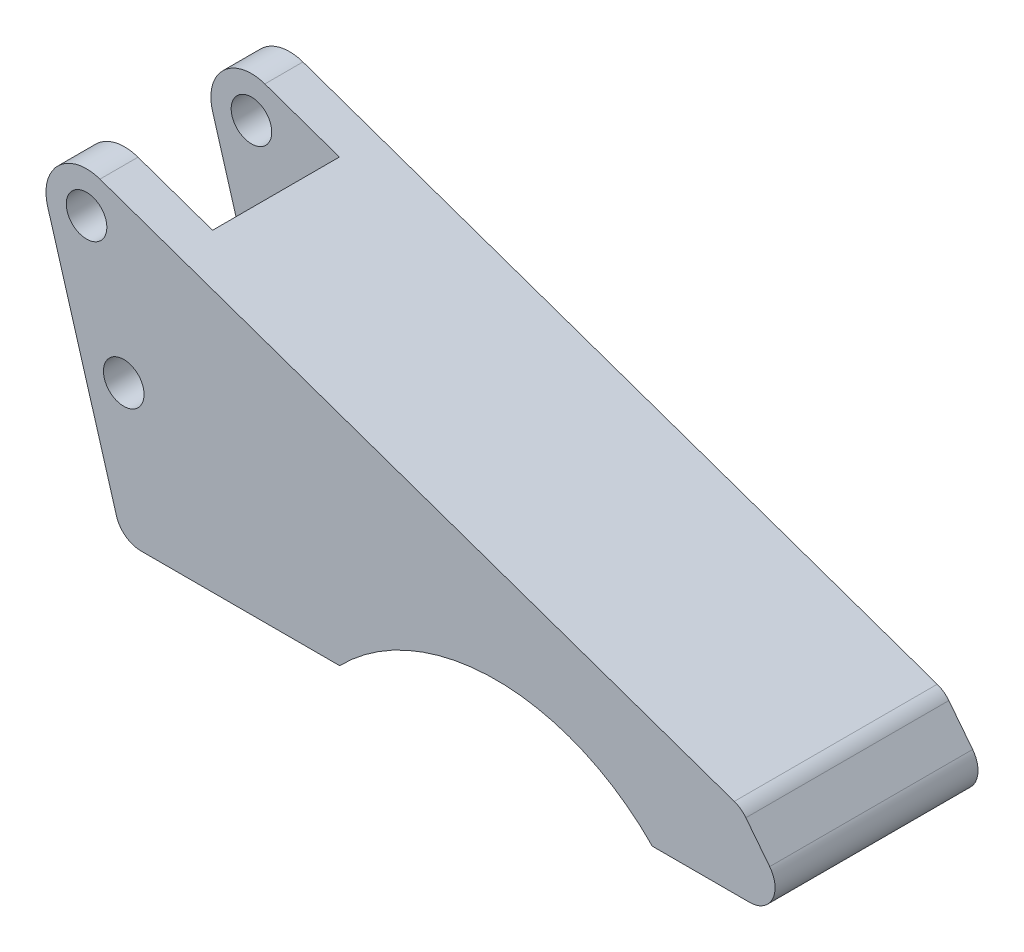
SolidWorks part; units mm, degrees
material "Plain Carbon Steel"
ref_plane "Front Plane" through (0, 0, 0) normal (0, 0, 1) x (1, 0, 0)
ref_plane "Top Plane" through (0, 0, 0) normal (0, 1, 0) x (1, 0, 0)
ref_plane "Right Plane" through (0, 0, 0) normal (1, 0, 0) x (0, 0, -1)
sketch "Jaw Profile Sketch" plane through (0, 0, 0) normal (0, 0, 1) x (1, 0, 0)
  line L0 (-39.1942, 0) -> (0, 0)
  line L1 (61.6117, 0) -> (80.8058, 0)
  line L2 (-47.2442, 59.4218) -> (77.7674, 15.7199)
  line L3 (80.0572, 14.0786) -> (84.7457, 8.0786)
  line L5 (-43.9901, 3.5861) -> (-57.5576, 49.6078)
  arc A0 (0, 0) -> (61.6117, 0) centre (30.8058, -30) cw
  circle A1 centre (-49.8842, 51.87) radius 4
  arc A2 (-47.2442, 59.4218) -> (-57.5576, 49.6078) centre (-49.8842, 51.87) ccw
  arc A3 (80.8058, 0) -> (84.7457, 8.0786) centre (80.8058, 5) ccw
  arc A4 (-39.1942, 0) -> (-43.9901, 3.5861) centre (-39.1942, 5) cw
  arc A5 (77.7674, 15.7199) -> (80.0572, 14.0786) centre (76.1174, 11) cw
  circle A6 centre (-42.5542, 27) radius 4
  dimension "D1" = 8
  dimension "D2" = 16
  dimension "D4" = 5
  dimension "D5" = 43
  dimension "D7" = 5
  dimension "D10" = 8
  dimension "D3" = 51.87
  dimension "D6" = 120
  dimension "D8" = 6
  dimension "D9" = 7.33
  dimension "D11" = 3.36
  dimension "D12" = 27
  dimension "D13" = 70
  dimension "D14" = 1.65
  dimension "D15" = 30
extrude "Jaw Plate 40mm" add sketch "Jaw Profile Sketch" along normal mid plane 40
sketch "Clevis Slot Sketch" plane through (0, 0, 0) normal (0, -1, 0) x (1, 0, 0)
  line L1 (-57.5576, 20) -> (-57.5576, -20) construction
  line L6 (-82.5576, -12.5) -> (-32.5576, -12.5)
  line L11 (-82.5576, -12.5) -> (-82.5576, 12.5)
  line L12 (-82.5576, 12.5) -> (-32.5576, 12.5)
  line L14 (-32.5576, -12.5) -> (-32.5576, 12.5)
  line L15 (-82.5576, -12.5) -> (-32.5576, 12.5) construction
  line L16 (-82.5576, 12.5) -> (-32.5576, -12.5) construction
  point P0 (-57.5576, 0)
  dimension "D1" = 25
  dimension "D2" = 50
extrude "Clevis Slot 25mm" cut sketch "Clevis Slot Sketch" against normal through all both and the other way through all
